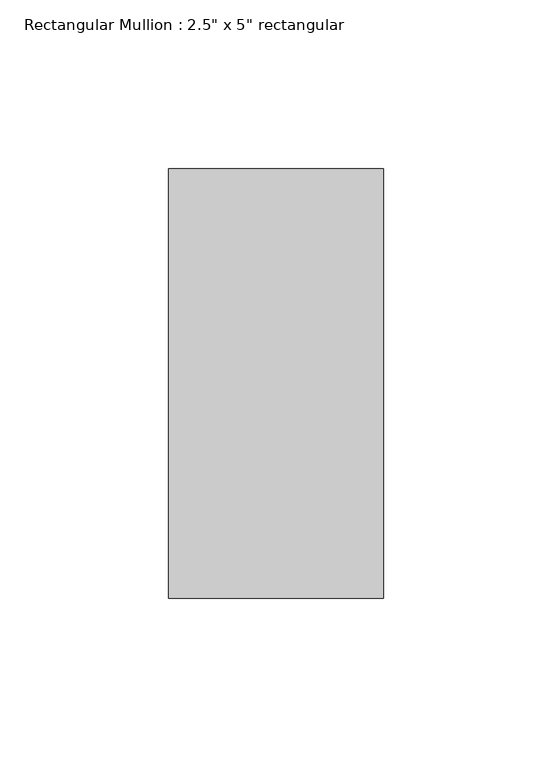
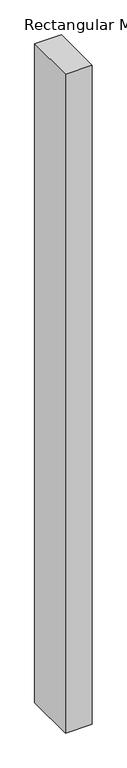
"""IFC4 building model written with IfcOpenShell, lengths in millimetres: member geometry."""

from ifc_helpers import new_model, si_unit, frame, origin, place, context, project, spatial, polyline, outline, extrude, source, transform, mapped, element, save


def member_c8b03bc0(model_context):
    return source(origin(), model_context, "Body", "SweptSolid", [
        extrude(outline(polyline([(0.0, 63.5), (0.0, -63.5), (-63.5, -63.5), (-63.5, 63.5), (0.0, 63.5)])), frame((0.0, 0.0, -1660.012385), z_axis=(0.0, 0.0, 1.0), x_axis=(1.0, 0.0, 0.0)), (0.0, 0.0, 1.0), 1660.012385),
    ])


if __name__ == "__main__":
    model = new_model("IFC4")
    model_context = context("Model", 3, world=origin())
    ifc_project = project(units=[si_unit("LENGTHUNIT", "METRE", prefix="MILLI")], contexts=[model_context])
    site = spatial("IfcSite", under=ifc_project)
    building = spatial("IfcBuilding", under=site)
    placement = place(None, origin())
    member_shape = member_c8b03bc0(model_context)
    element("IfcMember", 1, ObjectType="Rectangular Mullion : 2.5\" x 5\" rectangular", at=placement, inside=building, context=model_context, shape_type="MappedRepresentation", body=[
        mapped(member_shape, transform((0.0, 0.0, 0.0), x_axis=(1.0, 0.0, 0.0), y_axis=(0.0, 1.0, 0.0), z_axis=(0.0, 0.0, 1.0))),
    ])
    save(model, "model.ifc")

# Revit data of these elements
# Type "Rectangular Mullion : 2.5\" x 5\" rectangular"
#   built-in parameter 1007304 = 0.416667 (stored number, unit not read)
#   built-in parameter 1007301 = 0.104167 (stored number, unit not read)
#   built-in parameter 1007300 = 0.104167 (stored number, unit not read)
# Element 1 (IfcMember, "Rectangular Mullion : 2.5\" x 5\" rectangular")
#   Materials on its faces: "Aluminum"
# Materials
#   "Aluminum": class "Metal", colour RGB 247 247 247, transparency 0, Description = "Aluminum 6061", Cost = 0
